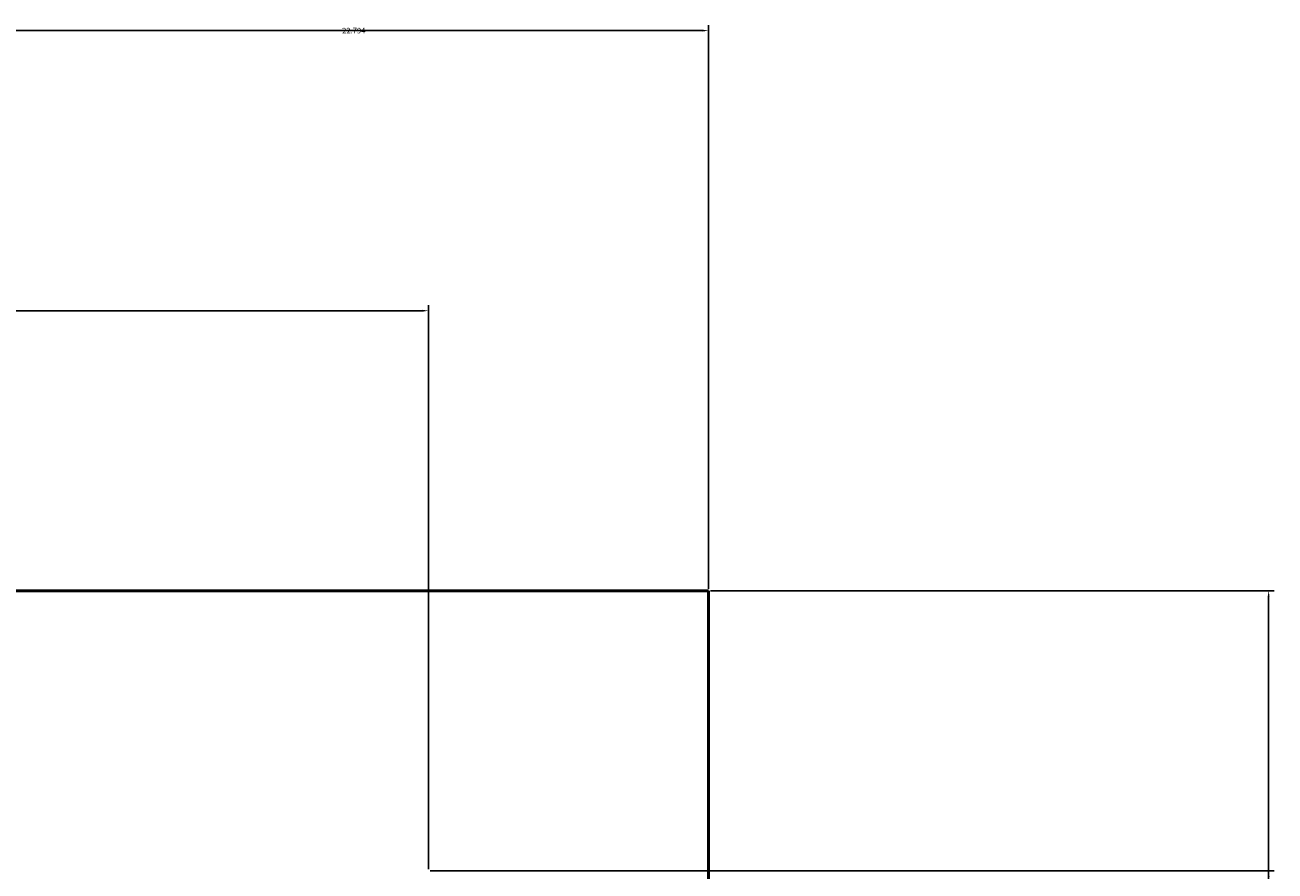
# Model space of a CAD drawing. Units: inches. Extents: x 2621 to 2849, y 2066 to 2463.
# Tile 28 of 28: x 2809 to 2849, y 2435 to 2463. Entities that reach past the tile are written whole.
import ezdxf

# ---------------------------------------------------------------- set-up
doc = ezdxf.new("R2010")
doc.units = ezdxf.units.IN
doc.layers.add('A-ANNO-DIMS', color=2, linetype='Continuous', lineweight=18)
doc.layers.add('A-WALL', color=7, linetype='Continuous', lineweight=50)
doc.styles.get("Standard").update_dxf_attribs({"font": 'arial.ttf'})
doc.dimstyles.get("Standard").update_dxf_attribs({"dimtxt": 0.18, "dimasz": 0.18, "dimexe": 0.18, "dimexo": 0.0625, "dimgap": 0.09, "dimtad": 0, "dimtih": 1, "dimtoh": 1, "dimdec": 4, "dimzin": 0, "dimdsep": 46, "dimtxsty": 'Standard', "dimcen": 0.09, "dimadec": 0, "dimazin": 0, "dimtfac": 1, "dimtdec": 4, "dimtofl": 0, "dimtmove": 0, "dimatfit": 3, "dimfxl": 1, "dimtolj": 1, "dimtzin": 0, "dimarcsym": 0})

# ---------------------------------------------------------------- blocks, each defined once
blk = doc.blocks.new('*D35')
at = {"layer": 'A-ANNO-DIMS', "color": 0, "lineweight": -2, "transparency": 16777216}
for p, q in [((2638.87, 2444.437), (2638.87, 2462.558)), ((2830.87, 2444.437), (2830.87, 2462.558)), ((2639.05, 2462.378), (2734.591, 2462.378)), ((2830.69, 2462.378), (2735.15, 2462.378))]:
    blk.add_line(p, q, dxfattribs=at)
at = {"layer": 'A-ANNO-DIMS', "color": 0, "transparency": 16777216}
for points in [[(2639.05, 2462.408), (2639.05, 2462.348), (2638.87, 2462.378)], [(2830.69, 2462.408), (2830.69, 2462.348), (2830.87, 2462.378)]]:
    blk.add_solid(points, dxfattribs=at)
at = {"layer": 'Defpoints', "color": 0, "transparency": 16777216}
for p in [(2830.87, 2462.378), (2638.87, 2444.375), (2830.87, 2444.375)]:
    blk.add_point(p, dxfattribs=at)
at = {"layer": 'A-ANNO-DIMS', "color": 0, "transparency": 16777216, "insert": (2734.87, 2462.378), "char_height": 0.18, "attachment_point": 5}
blk.add_mtext('\\A1;192', dxfattribs=at)
blk = doc.blocks.new('*D36')
at = {"layer": 'A-ANNO-DIMS', "color": 0, "lineweight": -2, "transparency": 16777216}
for p, q in [((2830.933, 2444.375), (2849.054, 2444.375)), ((2848.874, 2444.195), (2848.874, 2264.557)), ((2848.874, 2084.555), (2848.874, 2264.193)), ((2830.933, 2084.375), (2849.054, 2084.375))]:
    blk.add_line(p, q, dxfattribs=at)
at = {"layer": 'A-ANNO-DIMS', "color": 0, "transparency": 16777216}
for points in [[(2848.844, 2444.195), (2848.904, 2444.195), (2848.874, 2444.375)], [(2848.844, 2084.555), (2848.904, 2084.555), (2848.874, 2084.375)]]:
    blk.add_solid(points, dxfattribs=at)
at = {"layer": 'Defpoints', "color": 0, "transparency": 16777216}
for p in [(2830.87, 2444.375), (2848.874, 2444.375), (2830.87, 2084.375)]:
    blk.add_point(p, dxfattribs=at)
at = {"layer": 'A-ANNO-DIMS', "color": 0, "transparency": 16777216, "insert": (2848.874, 2264.375), "char_height": 0.18, "attachment_point": 5}
blk.add_mtext('\\A1;360', dxfattribs=at)
blk = doc.blocks.new('*D39')
at = {"layer": 'A-ANNO-DIMS', "color": 0, "lineweight": -2, "transparency": 16777216}
for p, q in [((2808.076, 2444.437), (2808.076, 2462.558)), ((2830.87, 2444.437), (2830.87, 2462.558)), ((2808.256, 2462.378), (2819.008, 2462.378)), ((2830.69, 2462.378), (2819.938, 2462.378))]:
    blk.add_line(p, q, dxfattribs=at)
at = {"layer": 'A-ANNO-DIMS', "color": 0, "transparency": 16777216}
for points in [[(2808.256, 2462.408), (2808.256, 2462.348), (2808.076, 2462.378)], [(2830.69, 2462.408), (2830.69, 2462.348), (2830.87, 2462.378)]]:
    blk.add_solid(points, dxfattribs=at)
at = {"layer": 'Defpoints', "color": 0, "transparency": 16777216}
for p in [(2830.87, 2462.378), (2808.076, 2444.375), (2830.87, 2444.375)]:
    blk.add_point(p, dxfattribs=at)
at = {"layer": 'A-ANNO-DIMS', "color": 0, "transparency": 16777216, "insert": (2819.473, 2462.378), "char_height": 0.18, "attachment_point": 5}
blk.add_mtext('\\A1;22.794', dxfattribs=at)
blk = doc.blocks.new('*D47')
at = {"layer": 'A-ANNO-DIMS', "color": 0, "lineweight": -2, "transparency": 16777216}
for p, q in [((2767.87, 2435.437), (2767.87, 2453.558)), ((2768.05, 2453.378), (2794.652, 2453.378)), ((2821.69, 2453.378), (2795.089, 2453.378)), ((2821.87, 2435.437), (2821.87, 2453.558))]:
    blk.add_line(p, q, dxfattribs=at)
at = {"layer": 'A-ANNO-DIMS', "color": 0, "transparency": 16777216}
for points in [[(2768.05, 2453.408), (2768.05, 2453.348), (2767.87, 2453.378)], [(2821.69, 2453.408), (2821.69, 2453.348), (2821.87, 2453.378)]]:
    blk.add_solid(points, dxfattribs=at)
at = {"layer": 'Defpoints', "color": 0, "transparency": 16777216}
for p in [(2821.87, 2453.378), (2767.87, 2435.375), (2821.87, 2435.375)]:
    blk.add_point(p, dxfattribs=at)
at = {"layer": 'A-ANNO-DIMS', "color": 0, "transparency": 16777216, "insert": (2794.87, 2453.378), "char_height": 0.18, "attachment_point": 5}
blk.add_mtext('\\A1;54', dxfattribs=at)
blk = doc.blocks.new('*D48')
at = {"layer": 'A-ANNO-DIMS', "color": 0, "lineweight": -2, "transparency": 16777216}
for p, q in [((2821.933, 2435.375), (2849.054, 2435.375)), ((2848.874, 2435.195), (2848.874, 2405.556)), ((2848.874, 2375.555), (2848.874, 2405.193)), ((2821.933, 2375.375), (2849.054, 2375.375))]:
    blk.add_line(p, q, dxfattribs=at)
at = {"layer": 'A-ANNO-DIMS', "color": 0, "transparency": 16777216}
for points in [[(2848.844, 2435.195), (2848.904, 2435.195), (2848.874, 2435.375)], [(2848.844, 2375.555), (2848.904, 2375.555), (2848.874, 2375.375)]]:
    blk.add_solid(points, dxfattribs=at)
at = {"layer": 'Defpoints', "color": 0, "transparency": 16777216}
for p in [(2821.87, 2435.375), (2848.874, 2435.375), (2821.87, 2375.375)]:
    blk.add_point(p, dxfattribs=at)
at = {"layer": 'A-ANNO-DIMS', "color": 0, "transparency": 16777216, "insert": (2848.874, 2405.375), "char_height": 0.18, "attachment_point": 5}
blk.add_mtext('\\A1;60', dxfattribs=at)

msp = doc.modelspace()

# ---------------------------------------------------------------- linework, layer by layer
at = {"layer": 'A-WALL'}
msp.add_lwpolyline([(2761.8701, 2084.3746), (2638.8701, 2084.3746), (2638.8701, 2444.3746), (2830.8701, 2444.3746), (2830.8701, 2084.3746), (2797.8701, 2084.3746)], dxfattribs=at)

# ---------------------------------------------------------------- dimensions: what is measured, and where the dimension line sits
at = {"layer": 'A-ANNO-DIMS'}
for base, p1, p2, override, picture, middle in [((2830.8701, 2462.3781), (2638.8701, 2444.3746), (2830.8701, 2444.3746), {"dimdec": 0, "dimlfac": 1, "dimrnd": 0, "dimzin": 0, "dimdsep": 46, "dimlunit": 2}, '*D35', (2734.8701, 2462.3781)), ((2830.8701, 2462.3781), (2808.0762, 2444.3746), (2830.8701, 2444.3746), {"dimdec": 3, "dimlfac": 1, "dimrnd": 0, "dimzin": 0, "dimdsep": 46, "dimlunit": 2}, '*D39', (2819.4732, 2462.3781)), ((2821.8701, 2453.3781), (2767.8701, 2435.3746), (2821.8701, 2435.3746), {"dimdec": 0, "dimlfac": 1, "dimrnd": 0, "dimzin": 0, "dimdsep": 46, "dimlunit": 2}, '*D47', (2794.8701, 2453.3781))]:
    dim = msp.add_linear_dim(base=base, p1=p1, p2=p2, dimstyle='Standard', override=override, dxfattribs=at)
    dim.commit()
    dim.dimension.update_dxf_attribs({"geometry": picture, "text_midpoint": middle})
for base, p1, p2, picture, middle in [((2848.8736, 2444.3746), (2830.8701, 2084.3746), (2830.8701, 2444.3746), '*D36', (2848.8736, 2264.3746)), ((2848.8736, 2435.3746), (2821.8701, 2375.3746), (2821.8701, 2435.3746), '*D48', (2848.8736, 2405.3746))]:
    dim = msp.add_linear_dim(base=base, p1=p1, p2=p2, angle=90, dimstyle='Standard', override={"dimdec": 0, "dimlfac": 1, "dimrnd": 0, "dimzin": 0, "dimdsep": 46, "dimlunit": 2}, dxfattribs=at)
    dim.commit()
    dim.dimension.update_dxf_attribs({"geometry": picture, "text_midpoint": middle})

doc.saveas('drawing.dxf')
